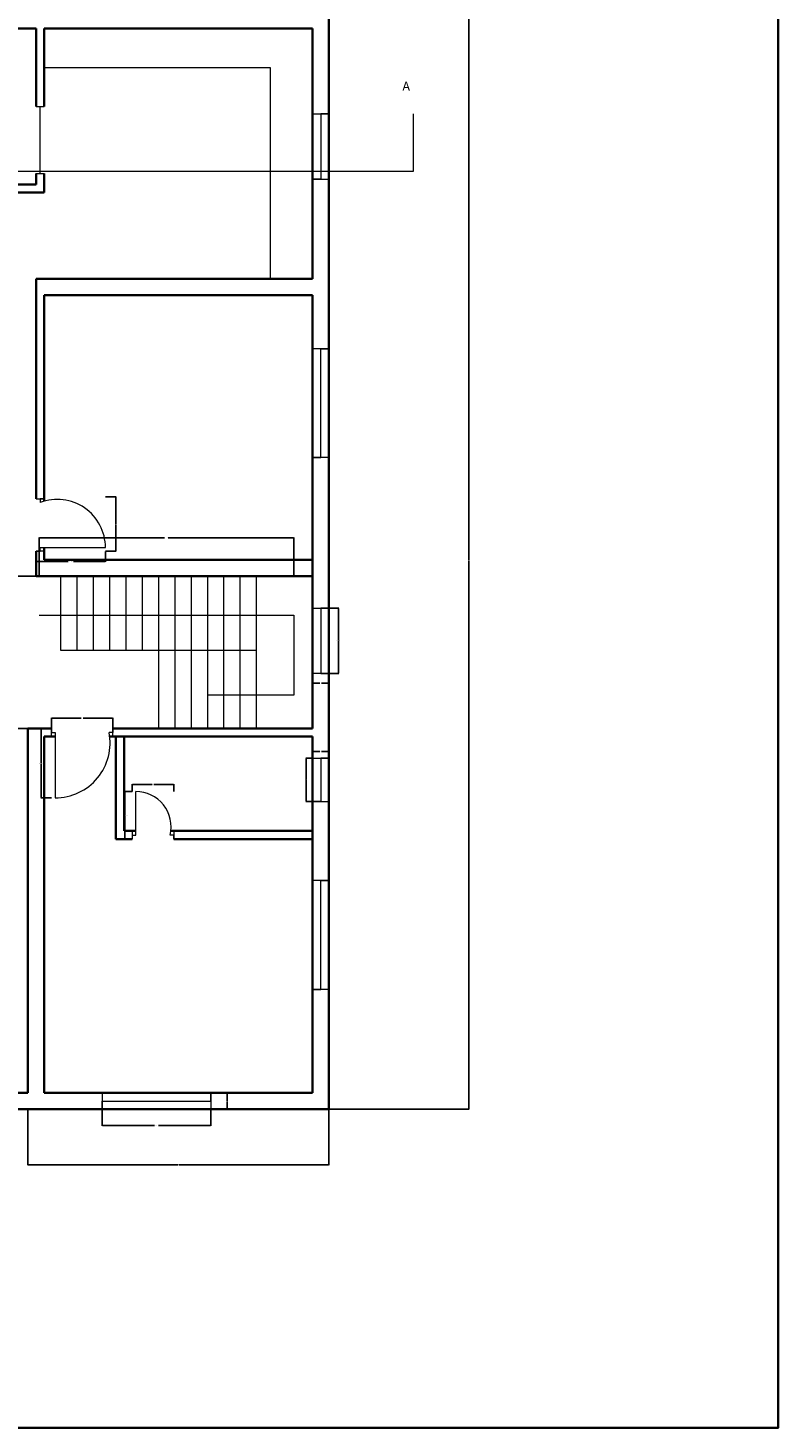
# Model space of a CAD drawing. Units: inches. Extents: x 1152 to 2588, y 1459 to 2618.
# Tile 16 of 17: x 2174 to 2588, y 1459 to 2231. Entities that reach past the tile are written whole.
import ezdxf

# ---------------------------------------------------------------- set-up
doc = ezdxf.new("R2010")
doc.units = ezdxf.units.IN
for name, color, linetype, lineweight in [('A-ANNO-DIMS', 2, 'Continuous', 18), ('A-ANNO-SYMB', 3, 'Continuous', 18), ('A-ANNO-TTLB', 7, 'Continuous', 35), ('A-DOOR', 4, 'Continuous', 18), ('A-FLOR-CASE', 30, 'Continuous', 18), ('A-FLOR-STRS', 3, 'Continuous', 18), ('A-GLAZ', 4, 'Continuous', 18), ('A-WALL', 7, 'Continuous', 35)]:
    doc.layers.add(name, color=color, linetype=linetype, lineweight=lineweight)
doc.styles.get("Standard").update_dxf_attribs({"font": 'arial.ttf'})
doc.dimstyles.get("Standard").update_dxf_attribs({"dimtxt": 0.18, "dimasz": 0.18, "dimexe": 0.18, "dimexo": 0.0625, "dimgap": 0.09, "dimtad": 0, "dimtih": 1, "dimtoh": 1, "dimdec": 4, "dimzin": 0, "dimdsep": 46, "dimtxsty": 'Standard', "dimcen": 0.09, "dimadec": 0, "dimazin": 0, "dimtfac": 1, "dimtdec": 4, "dimtofl": 0, "dimtmove": 0, "dimatfit": 3, "dimfxl": 1, "dimtolj": 1, "dimtzin": 0, "dimarcsym": 0})

# ---------------------------------------------------------------- blocks, each defined once
blk = doc.blocks.new('DOOR-24-ENSUITE')
for p, q in [((2, 2.25), (2, 26.25)), ((0, 4.5), (0, 0)), ((0, 2.25), (2, 2.25)), ((23, 2.25), (21, 2.25)), ((23, 4.5), (23, 0)), ((23, 0), (23, 2.25)), ((23, 2.25), (23, 2.25)), ((0, 0), (0, 0))]:
    blk.add_line(p, q)
blk.add_arc((2, 6.73), 19.52, 346.72099, 90)
blk = doc.blocks.new('DOOR-36-STORE')
for p, q in [((0, 28.88), (4.5, 28.88)), ((4.5, 28.88), (2.25, 28.88)), ((2.25, 28.88), (2.25, 26.88)), ((4.5, 0), (0, 0)), ((0, 0), (2.25, 0)), ((2.25, 0), (2.25, 2)), ((2.25, 2), (38.25, 2))]:
    blk.add_line(p, q)
blk.add_arc((11.65, 2), 26.6, 0, 110.70701)
blk = doc.blocks.new('DOOR-36-HALL')
for p, q in [((0, 33.75), (0, 38.25)), ((0, 38.25), (0, 36)), ((0, 36), (2, 36)), ((2, 36), (2, 0)), ((33.77, 36), (31.77, 36)), ((33.77, 33.75), (33.77, 38.25)), ((33.77, 38.25), (33.77, 36))]:
    blk.add_line(p, q)
blk.add_arc((2, 30.31), 30.31, 270, 10.81625)
blk = doc.blocks.new('DOOR-STORE-OPENING')
for p, q in [((0, 36.9), (4.5, 36.9)), ((2.25, 0), (2.25, 36.9)), ((0, 0), (4.5, 0))]:
    blk.add_line(p, q)
blk = doc.blocks.new('WIN-60-EXT')
for p, q in [((0, 9), (0, 0)), ((60, 4.5), (60, 9)), ((60, 9), (60, 0)), ((0, 0), (0, 4.5)), ((0, 4.5), (60, 4.5))]:
    blk.add_line(p, q)
blk = doc.blocks.new('WIN-36')
for p, q in [((0, 36), (9, 36)), ((9, 36), (4.5, 36)), ((4.5, 36), (4.5, 0)), ((4.5, 0), (0, 0)), ((0, 0), (9, 0))]:
    blk.add_line(p, q)
blk = doc.blocks.new('WIN-24-BATH-EAST')
for p, q in [((0, 24), (9, 24)), ((9, 24), (4.5, 24)), ((4.5, 24), (4.5, 0)), ((4.5, 0), (0, 0)), ((0, 0), (9, 0))]:
    blk.add_line(p, q)
blk = doc.blocks.new('WIN-36-STAIR')
for p, q in [((0, 36), (9, 36)), ((9, 36), (4.5, 36)), ((4.5, 36), (4.5, 0)), ((9, 0), (0, 0)), ((4.5, 0), (9, 0))]:
    blk.add_line(p, q)
blk = doc.blocks.new('STAIR-RETURN')
for p, q in [((12.04, 42.95), (12.04, 84)), ((21.04, 42.95), (21.04, 84)), ((30.04, 42.95), (30.04, 84)), ((39.04, 42.95), (39.04, 84)), ((48.04, 42.95), (48.04, 84)), ((57.04, 42.95), (57.04, 84)), ((66.04, 0), (66.04, 84)), ((75.04, 0), (75.04, 84)), ((84.04, 0), (84.04, 84)), ((93.04, 0), (93.04, 84)), ((102.04, 0), (102.04, 84)), ((111.04, 0), (111.04, 84)), ((120.04, 0), (120.04, 84)), ((0, 62.54), (140.6, 62.54)), ((140.6, 62.54), (140.6, 18.44)), ((120.04, 42.95), (12.04, 42.95)), ((140.6, 18.44), (93.04, 18.44))]:
    blk.add_line(p, q)
blk = doc.blocks.new('COUNTER-KITCHEN-L')
for p, q in [((0, 116.5), (124.66, 116.5)), ((124.66, 116.5), (124.66, 0))]:
    blk.add_line(p, q)
blk = doc.blocks.new('*D26')
at = {"layer": 'A-ANNO-DIMS', "color": 0, "lineweight": -2, "transparency": 16777216}
for p, q in [((2214.75, 1634.98), (2214.75, 1625.87)), ((2274.75, 1634.98), (2274.75, 1625.87)), ((2214.93, 1626.05), (2243.6, 1626.05)), ((2274.57, 1626.05), (2245.9, 1626.05))]:
    blk.add_line(p, q, dxfattribs=at)
at = {"layer": 'A-ANNO-DIMS', "color": 0, "transparency": 16777216}
for points in [[(2214.93, 1626.08), (2214.93, 1626.02), (2214.75, 1626.05)], [(2274.57, 1626.08), (2274.57, 1626.02), (2274.75, 1626.05)]]:
    blk.add_solid(points, dxfattribs=at)
at = {"layer": 'Defpoints', "color": 0, "transparency": 16777216}
for p in [(2214.75, 1635.05), (2274.75, 1635.05), (2274.75, 1626.05)]:
    blk.add_point(p, dxfattribs=at)
at = {"layer": 'A-ANNO-DIMS', "color": 0, "transparency": 16777216, "insert": (2244.75, 1626.05), "char_height": 0.18, "attachment_point": 5}
blk.add_mtext('\\A1;EXT. WIN. 60 TYP.', dxfattribs=at)
blk = doc.blocks.new('*D27')
at = {"layer": 'A-ANNO-DIMS', "color": 0, "lineweight": -2, "transparency": 16777216}
for p, q in [((2274.81, 1644.05), (2283.93, 1644.05)), ((2283.75, 1643.87), (2283.75, 1639.73)), ((2283.75, 1635.23), (2283.75, 1639.36)), ((2274.81, 1635.05), (2283.93, 1635.05))]:
    blk.add_line(p, q, dxfattribs=at)
at = {"layer": 'A-ANNO-DIMS', "color": 0, "transparency": 16777216}
for points in [[(2283.72, 1643.87), (2283.78, 1643.87), (2283.75, 1644.05)], [(2283.72, 1635.23), (2283.78, 1635.23), (2283.75, 1635.05)]]:
    blk.add_solid(points, dxfattribs=at)
at = {"layer": 'Defpoints', "color": 0, "transparency": 16777216}
for p in [(2274.75, 1644.05), (2283.75, 1644.05), (2274.75, 1635.05)]:
    blk.add_point(p, dxfattribs=at)
at = {"layer": 'A-ANNO-DIMS', "color": 0, "transparency": 16777216, "insert": (2283.75, 1639.55), "char_height": 0.18, "attachment_point": 5}
blk.add_mtext('\\A1;9 TYP.', dxfattribs=at)
blk = doc.blocks.new('*D38')
at = {"layer": 'A-ANNO-DIMS', "color": 0, "lineweight": -2, "transparency": 16777216}
for p, q in [((2231.28, 1810.3), (2227.22, 1810.3)), ((2227.4, 1810.12), (2227.4, 1797.35)), ((2227.4, 1784.23), (2227.4, 1796.99)), ((2231.28, 1784.05), (2227.22, 1784.05))]:
    blk.add_line(p, q, dxfattribs=at)
at = {"layer": 'A-ANNO-DIMS', "color": 0, "transparency": 16777216}
for points in [[(2227.37, 1810.12), (2227.43, 1810.12), (2227.4, 1810.3)], [(2227.37, 1784.23), (2227.43, 1784.23), (2227.4, 1784.05)]]:
    blk.add_solid(points, dxfattribs=at)
at = {"layer": 'Defpoints', "color": 0, "transparency": 16777216}
for p in [(2227.4, 1810.3), (2231.34, 1810.3), (2231.34, 1784.05)]:
    blk.add_point(p, dxfattribs=at)
at = {"layer": 'A-ANNO-DIMS', "color": 0, "transparency": 16777216, "insert": (2227.4, 1797.17), "char_height": 0.18, "attachment_point": 5}
blk.add_mtext('\\A1;ENSUITE DOOR 26 TYP.', dxfattribs=at)
blk = doc.blocks.new('*D39')
at = {"layer": 'A-ANNO-DIMS', "color": 0, "lineweight": -2, "transparency": 16777216}
for p, q in [((2231.34, 1810.36), (2231.34, 1814.41)), ((2231.52, 1814.23), (2242.31, 1814.23)), ((2254.15, 1814.23), (2243.36, 1814.23)), ((2254.33, 1810.36), (2254.33, 1814.41))]:
    blk.add_line(p, q, dxfattribs=at)
at = {"layer": 'A-ANNO-DIMS', "color": 0, "transparency": 16777216}
for points in [[(2231.52, 1814.26), (2231.52, 1814.2), (2231.34, 1814.23)], [(2254.15, 1814.26), (2254.15, 1814.2), (2254.33, 1814.23)]]:
    blk.add_solid(points, dxfattribs=at)
at = {"layer": 'Defpoints', "color": 0, "transparency": 16777216}
for p in [(2254.33, 1814.23), (2231.34, 1810.3), (2254.33, 1810.3)]:
    blk.add_point(p, dxfattribs=at)
at = {"layer": 'A-ANNO-DIMS', "color": 0, "transparency": 16777216, "insert": (2242.84, 1814.23), "char_height": 0.18, "attachment_point": 5}
blk.add_mtext('\\A1;23 TYP.', dxfattribs=at)
blk = doc.blocks.new('*D46')
at = {"layer": 'A-ANNO-DIMS', "color": 0, "lineweight": -2, "transparency": 16777216}
for p, q in [((2178.38, 1942.71), (2178.38, 1936.85)), ((2216.63, 1942.71), (2216.63, 1936.85)), ((2178.56, 1937.03), (2196.1, 1937.03)), ((2216.45, 1937.03), (2198.92, 1937.03))]:
    blk.add_line(p, q, dxfattribs=at)
at = {"layer": 'A-ANNO-DIMS', "color": 0, "transparency": 16777216}
for points in [[(2178.56, 1937.06), (2178.56, 1937), (2178.38, 1937.03)], [(2216.45, 1937.06), (2216.45, 1937), (2216.63, 1937.03)]]:
    blk.add_solid(points, dxfattribs=at)
at = {"layer": 'Defpoints', "color": 0, "transparency": 16777216}
for p in [(2178.38, 1942.77), (2216.63, 1942.77), (2216.63, 1937.03)]:
    blk.add_point(p, dxfattribs=at)
at = {"layer": 'A-ANNO-DIMS', "color": 0, "transparency": 16777216, "insert": (2197.51, 1937.03), "char_height": 0.18, "attachment_point": 5}
blk.add_mtext('\\A1;STORE DOOR 38 TYP.', dxfattribs=at)
blk = doc.blocks.new('*D47')
at = {"layer": 'A-ANNO-DIMS', "color": 0, "lineweight": -2, "transparency": 16777216}
for p, q in [((2216.7, 1972.74), (2222.55, 1972.74)), ((2222.37, 1972.56), (2222.37, 1957.94)), ((2222.37, 1942.95), (2222.37, 1957.57)), ((2216.7, 1942.77), (2222.55, 1942.77))]:
    blk.add_line(p, q, dxfattribs=at)
at = {"layer": 'A-ANNO-DIMS', "color": 0, "transparency": 16777216}
for points in [[(2222.34, 1972.56), (2222.4, 1972.56), (2222.37, 1972.74)], [(2222.34, 1942.95), (2222.4, 1942.95), (2222.37, 1942.77)]]:
    blk.add_solid(points, dxfattribs=at)
at = {"layer": 'Defpoints', "color": 0, "transparency": 16777216}
for p in [(2216.63, 1972.74), (2222.37, 1972.74), (2216.63, 1942.77)]:
    blk.add_point(p, dxfattribs=at)
at = {"layer": 'A-ANNO-DIMS', "color": 0, "transparency": 16777216, "insert": (2222.37, 1957.76), "char_height": 0.18, "attachment_point": 5}
blk.add_mtext('\\A1;30 TYP.', dxfattribs=at)
blk = doc.blocks.new('*D48')
at = {"layer": 'A-ANNO-DIMS', "color": 0, "lineweight": -2, "transparency": 16777216}
for p, q in [((2186.81, 1845.05), (2180.95, 1845.05)), ((2181.13, 1844.87), (2181.13, 1826.1)), ((2181.13, 1806.98), (2181.13, 1825.74)), ((2186.81, 1806.8), (2180.95, 1806.8))]:
    blk.add_line(p, q, dxfattribs=at)
at = {"layer": 'A-ANNO-DIMS', "color": 0, "transparency": 16777216}
for points in [[(2181.1, 1844.87), (2181.16, 1844.87), (2181.13, 1845.05)], [(2181.1, 1806.98), (2181.16, 1806.98), (2181.13, 1806.8)]]:
    blk.add_solid(points, dxfattribs=at)
at = {"layer": 'Defpoints', "color": 0, "transparency": 16777216}
for p in [(2181.13, 1845.05), (2186.87, 1845.05), (2186.87, 1806.8)]:
    blk.add_point(p, dxfattribs=at)
at = {"layer": 'A-ANNO-DIMS', "color": 0, "transparency": 16777216, "insert": (2181.13, 1825.92), "char_height": 0.18, "attachment_point": 5}
blk.add_mtext('\\A1;HALL DOOR 38 TYP.', dxfattribs=at)
blk = doc.blocks.new('*D49')
at = {"layer": 'A-ANNO-DIMS', "color": 0, "lineweight": -2, "transparency": 16777216}
for p, q in [((2186.87, 1845.11), (2186.87, 1850.96)), ((2187.05, 1850.78), (2203.23, 1850.78)), ((2220.46, 1850.78), (2204.29, 1850.78)), ((2220.64, 1845.11), (2220.64, 1850.96))]:
    blk.add_line(p, q, dxfattribs=at)
at = {"layer": 'A-ANNO-DIMS', "color": 0, "transparency": 16777216}
for points in [[(2187.05, 1850.81), (2187.05, 1850.75), (2186.87, 1850.78)], [(2220.46, 1850.81), (2220.46, 1850.75), (2220.64, 1850.78)]]:
    blk.add_solid(points, dxfattribs=at)
at = {"layer": 'Defpoints', "color": 0, "transparency": 16777216}
for p in [(2186.87, 1845.05), (2220.64, 1850.78), (2220.64, 1845.05)]:
    blk.add_point(p, dxfattribs=at)
at = {"layer": 'A-ANNO-DIMS', "color": 0, "transparency": 16777216, "insert": (2203.76, 1850.78), "char_height": 0.18, "attachment_point": 5}
blk.add_mtext('\\A1;34 TYP.', dxfattribs=at)
blk = doc.blocks.new('*D58')
at = {"layer": 'A-ANNO-DIMS', "color": 0, "lineweight": -2, "transparency": 16777216}
for p, q in [((2330.82, 1828.76), (2327.1, 1828.76)), ((2327.28, 1828.58), (2327.28, 1816.94)), ((2327.28, 1804.94), (2327.28, 1816.58)), ((2330.82, 1804.76), (2327.1, 1804.76))]:
    blk.add_line(p, q, dxfattribs=at)
at = {"layer": 'A-ANNO-DIMS', "color": 0, "transparency": 16777216}
for points in [[(2327.25, 1828.58), (2327.31, 1828.58), (2327.28, 1828.76)], [(2327.25, 1804.94), (2327.31, 1804.94), (2327.28, 1804.76)]]:
    blk.add_solid(points, dxfattribs=at)
at = {"layer": 'Defpoints', "color": 0, "transparency": 16777216}
for p in [(2327.28, 1828.76), (2330.88, 1828.76), (2330.88, 1804.76)]:
    blk.add_point(p, dxfattribs=at)
at = {"layer": 'A-ANNO-DIMS', "color": 0, "transparency": 16777216, "insert": (2327.28, 1816.76), "char_height": 0.18, "attachment_point": 5}
blk.add_mtext('\\A1;WIN. 24 TYP.', dxfattribs=at)
blk = doc.blocks.new('*D59')
at = {"layer": 'A-ANNO-DIMS', "color": 0, "lineweight": -2, "transparency": 16777216}
for p, q in [((2330.88, 1828.82), (2330.88, 1832.54)), ((2331.06, 1832.36), (2334.93, 1832.36)), ((2339.7, 1832.36), (2335.84, 1832.36)), ((2339.88, 1828.82), (2339.88, 1832.54))]:
    blk.add_line(p, q, dxfattribs=at)
at = {"layer": 'A-ANNO-DIMS', "color": 0, "transparency": 16777216}
for points in [[(2331.06, 1832.39), (2331.06, 1832.33), (2330.88, 1832.36)], [(2339.7, 1832.39), (2339.7, 1832.33), (2339.88, 1832.36)]]:
    blk.add_solid(points, dxfattribs=at)
at = {"layer": 'Defpoints', "color": 0, "transparency": 16777216}
for p in [(2339.88, 1832.36), (2330.88, 1828.76), (2339.88, 1828.76)]:
    blk.add_point(p, dxfattribs=at)
at = {"layer": 'A-ANNO-DIMS', "color": 0, "transparency": 16777216, "insert": (2335.38, 1832.36), "char_height": 0.18, "attachment_point": 5}
blk.add_mtext('\\A1;9 TYP.', dxfattribs=at)
blk = doc.blocks.new('*D62')
at = {"layer": 'A-ANNO-DIMS', "color": 0, "lineweight": -2, "transparency": 16777216}
for p, q in [((2339.95, 1911.36), (2345.46, 1911.36)), ((2345.28, 1911.18), (2345.28, 1893.54)), ((2345.28, 1875.54), (2345.28, 1893.17)), ((2339.95, 1875.36), (2345.46, 1875.36))]:
    blk.add_line(p, q, dxfattribs=at)
at = {"layer": 'A-ANNO-DIMS', "color": 0, "transparency": 16777216}
for points in [[(2345.25, 1911.18), (2345.31, 1911.18), (2345.28, 1911.36)], [(2345.25, 1875.54), (2345.31, 1875.54), (2345.28, 1875.36)]]:
    blk.add_solid(points, dxfattribs=at)
at = {"layer": 'Defpoints', "color": 0, "transparency": 16777216}
for p in [(2339.88, 1911.36), (2345.28, 1911.36), (2339.88, 1875.36)]:
    blk.add_point(p, dxfattribs=at)
at = {"layer": 'A-ANNO-DIMS', "color": 0, "transparency": 16777216, "insert": (2345.28, 1893.36), "char_height": 0.18, "attachment_point": 5}
blk.add_mtext('\\A1;STAIR WIN. 36 TYP.', dxfattribs=at)
blk = doc.blocks.new('*D63')
at = {"layer": 'A-ANNO-DIMS', "color": 0, "lineweight": -2, "transparency": 16777216}
for p, q in [((2330.88, 1875.29), (2330.88, 1869.78)), ((2331.06, 1869.96), (2334.93, 1869.96)), ((2339.7, 1869.96), (2335.84, 1869.96)), ((2339.88, 1875.29), (2339.88, 1869.78))]:
    blk.add_line(p, q, dxfattribs=at)
at = {"layer": 'A-ANNO-DIMS', "color": 0, "transparency": 16777216}
for points in [[(2331.06, 1869.99), (2331.06, 1869.93), (2330.88, 1869.96)], [(2339.7, 1869.99), (2339.7, 1869.93), (2339.88, 1869.96)]]:
    blk.add_solid(points, dxfattribs=at)
at = {"layer": 'Defpoints', "color": 0, "transparency": 16777216}
for p in [(2330.88, 1875.36), (2339.88, 1875.36), (2339.88, 1869.96)]:
    blk.add_point(p, dxfattribs=at)
at = {"layer": 'A-ANNO-DIMS', "color": 0, "transparency": 16777216, "insert": (2335.38, 1869.96), "char_height": 0.18, "attachment_point": 5}
blk.add_mtext('\\A1;9 TYP.', dxfattribs=at)
blk = doc.blocks.new('*D66')
at = {"layer": 'A-ANNO-DIMS', "color": 0, "lineweight": -2, "transparency": 16777216}
for p, q in [((2179.99, 1929.11), (2179.99, 1950.32)), ((2180.17, 1950.14), (2249.29, 1950.14)), ((2320.41, 1950.14), (2251.29, 1950.14)), ((2320.59, 1929.11), (2320.59, 1950.32))]:
    blk.add_line(p, q, dxfattribs=at)
at = {"layer": 'A-ANNO-DIMS', "color": 0, "transparency": 16777216}
for points in [[(2180.17, 1950.17), (2180.17, 1950.11), (2179.99, 1950.14)], [(2320.41, 1950.17), (2320.41, 1950.11), (2320.59, 1950.14)]]:
    blk.add_solid(points, dxfattribs=at)
at = {"layer": 'Defpoints', "color": 0, "transparency": 16777216}
for p in [(2320.59, 1950.14), (2179.99, 1929.05), (2320.59, 1929.05)]:
    blk.add_point(p, dxfattribs=at)
at = {"layer": 'A-ANNO-DIMS', "color": 0, "transparency": 16777216, "insert": (2250.29, 1950.14), "char_height": 0.18, "attachment_point": 5}
blk.add_mtext('\\A1;STAIR 141 TYP.', dxfattribs=at)
blk = doc.blocks.new('*D67')
at = {"layer": 'A-ANNO-DIMS', "color": 0, "lineweight": -2, "transparency": 16777216}
for p, q in [((2179.93, 1929.05), (2158.72, 1929.05)), ((2158.9, 1928.87), (2158.9, 1887.23)), ((2158.9, 1845.23), (2158.9, 1886.86)), ((2179.93, 1845.05), (2158.72, 1845.05))]:
    blk.add_line(p, q, dxfattribs=at)
at = {"layer": 'A-ANNO-DIMS', "color": 0, "transparency": 16777216}
for points in [[(2158.87, 1928.87), (2158.93, 1928.87), (2158.9, 1929.05)], [(2158.87, 1845.23), (2158.93, 1845.23), (2158.9, 1845.05)]]:
    blk.add_solid(points, dxfattribs=at)
at = {"layer": 'Defpoints', "color": 0, "transparency": 16777216}
for p in [(2158.9, 1929.05), (2179.99, 1929.05), (2179.99, 1845.05)]:
    blk.add_point(p, dxfattribs=at)
at = {"layer": 'A-ANNO-DIMS', "color": 0, "transparency": 16777216, "insert": (2158.9, 1887.05), "char_height": 0.18, "attachment_point": 5}
blk.add_mtext('\\A1;84 TYP.', dxfattribs=at)
blk = doc.blocks.new('*D78')
at = {"layer": 'A-ANNO-DIMS', "color": 0, "lineweight": -2, "transparency": 16777216}
for p, q in [((2339.95, 2240.05), (2417.36, 2240.05)), ((2417.18, 2239.87), (2417.18, 1937.73)), ((2417.18, 1635.23), (2417.18, 1937.36)), ((2339.95, 1635.05), (2417.36, 1635.05))]:
    blk.add_line(p, q, dxfattribs=at)
at = {"layer": 'A-ANNO-DIMS', "color": 0, "transparency": 16777216}
for points in [[(2417.15, 2239.87), (2417.21, 2239.87), (2417.18, 2240.05)], [(2417.15, 1635.23), (2417.21, 1635.23), (2417.18, 1635.05)]]:
    blk.add_solid(points, dxfattribs=at)
at = {"layer": 'Defpoints', "color": 0, "transparency": 16777216}
for p in [(2339.88, 2240.05), (2417.18, 2240.05), (2339.88, 1635.05)]:
    blk.add_point(p, dxfattribs=at)
at = {"layer": 'A-ANNO-DIMS', "color": 0, "transparency": 16777216, "insert": (2417.18, 1937.55), "char_height": 0.18, "attachment_point": 5}
blk.add_mtext('\\A1;605', dxfattribs=at)
blk = doc.blocks.new('*D87')
at = {"layer": 'A-ANNO-DIMS', "color": 0, "lineweight": -2, "transparency": 16777216}
for p, q in [((2173.88, 1634.98), (2173.88, 1604.27)), ((2339.88, 1634.98), (2339.88, 1604.27)), ((2174.06, 1604.45), (2256.6, 1604.45)), ((2339.7, 1604.45), (2257.16, 1604.45))]:
    blk.add_line(p, q, dxfattribs=at)
at = {"layer": 'A-ANNO-DIMS', "color": 0, "transparency": 16777216}
for points in [[(2174.06, 1604.48), (2174.06, 1604.42), (2173.88, 1604.45)], [(2339.7, 1604.48), (2339.7, 1604.42), (2339.88, 1604.45)]]:
    blk.add_solid(points, dxfattribs=at)
at = {"layer": 'Defpoints', "color": 0, "transparency": 16777216}
for p in [(2173.88, 1635.05), (2339.88, 1635.05), (2339.88, 1604.45)]:
    blk.add_point(p, dxfattribs=at)
at = {"layer": 'A-ANNO-DIMS', "color": 0, "transparency": 16777216, "insert": (2256.88, 1604.45), "char_height": 0.18, "attachment_point": 5}
blk.add_mtext('\\A1;166', dxfattribs=at)

msp = doc.modelspace()

# ---------------------------------------------------------------- linework, layer by layer
at = {"layer": 'A-ANNO-SYMB'}
for p, q in [((2386.5775, 2152.3313), (2386.5775, 2183.955)), ((1847.169, 2152.3313), (2386.5775, 2152.3313))]:
    msp.add_line(p, q, dxfattribs=at)
at = {"layer": 'A-ANNO-TTLB'}
msp.add_lwpolyline([(1152.3215, 2617.6685), (2587.6987, 2617.6685), (2587.6987, 1459.3148), (1152.3215, 1459.3148)], close=True, dxfattribs=at)
at = {"layer": 'A-WALL'}
for p, q in [((2339.8841, 2240.0458), (2339.8841, 1635.0458)), ((2130.3841, 2231.0458), (2178.3841, 2231.0458)), ((2178.3841, 2231.0458), (2178.3841, 2188.0458)), ((2182.8841, 2231.0458), (2330.8841, 2231.0458)), ((2182.8841, 2231.0458), (2182.8841, 2188.0458)), ((2330.8841, 2231.0458), (2330.8841, 2093.0458)), ((2178.3841, 2151.1471), (2178.3841, 2145.0458)), ((2182.8841, 2151.1471), (2182.8841, 2140.5458)), ((2130.3841, 2145.0458), (2178.3841, 2145.0458)), ((2130.3841, 2140.5458), (2178.3841, 2140.5458)), ((2178.3841, 2140.5458), (2182.8841, 2140.5458)), ((2178.3841, 2093.0458), (2178.3841, 1971.6501)), ((2182.8841, 2093.0458), (2178.3841, 2093.0458)), ((2182.8841, 2093.0458), (2330.8841, 2093.0458)), ((2182.8841, 2084.0458), (2330.8841, 2084.0458)), ((2182.8841, 2084.0458), (2182.8841, 1970.3879)), ((2330.8841, 2084.0458), (2330.8841, 1845.0458)), ((2178.3841, 1942.7722), (2178.3841, 1929.0458)), ((2182.8841, 1944.7722), (2182.8841, 1938.0458)), ((2182.8841, 1938.0458), (2330.8841, 1938.0458)), ((2178.3841, 1929.0458), (2330.8841, 1929.0458)), ((2173.8841, 1845.0458), (2182.8841, 1845.0458)), ((2173.8841, 1840.5831), (2173.8841, 1845.0458)), ((2182.8841, 1845.0458), (2186.8711, 1845.0458)), ((2220.6443, 1845.0458), (2330.8841, 1845.0458)), ((2173.8841, 1644.0458), (2173.8841, 1840.5831)), ((2182.8841, 1840.5458), (2188.8711, 1840.5458)), ((2182.8841, 1840.5458), (2182.8841, 1644.0458)), ((2218.9872, 1840.5458), (2330.8841, 1840.5458)), ((2226.8841, 1840.5458), (2222.3841, 1840.5458)), ((2222.3841, 1840.5458), (2222.3841, 1788.5458)), ((2226.8841, 1788.5458), (2226.8841, 1840.5458)), ((2330.8841, 1840.5458), (2330.8841, 1644.0458)), ((2330.8841, 1840.5458), (2330.8841, 1788.5458)), ((2222.3841, 1788.5458), (2222.3841, 1784.0458)), ((2222.3841, 1784.0458), (2231.3375, 1784.0458)), ((2233.3375, 1788.5458), (2226.8841, 1788.5458)), ((2330.8841, 1788.5458), (2252.7264, 1788.5458)), ((2254.3327, 1784.0458), (2330.8841, 1784.0458)), ((2073.5339, 1644.0458), (2173.8841, 1644.0458)), ((2182.8841, 1644.0458), (2330.8841, 1644.0458)), ((2075.5339, 1635.0458), (2339.8841, 1635.0458)), ((2182.8841, 1635.0458), (2173.8841, 1635.0458))]:
    msp.add_line(p, q, dxfattribs=at)

# ---------------------------------------------------------------- block references
at = {"layer": 'A-DOOR'}
for name, p in [('DOOR-STORE-OPENING', (2178.3846, 2151.147)), ('DOOR-36-STORE', (2178.3846, 1942.772)), ('DOOR-36-HALL', (2186.8716, 1806.796)), ('DOOR-24-ENSUITE', (2231.3376, 1784.046))]:
    msp.add_blockref(name, p, dxfattribs=at)
at = {"layer": 'A-FLOR-CASE'}
msp.add_blockref('COUNTER-KITCHEN-L', (2182.8846, 2093.046), dxfattribs=at)
at = {"layer": 'A-FLOR-STRS'}
msp.add_blockref('STAIR-RETURN', (2179.9916, 1845.046), dxfattribs=at)
at = {"layer": 'A-GLAZ'}
for name, p in [('WIN-36', (2330.8846, 2147.9727)), ('WIN-36-STAIR', (2330.8846, 1875.356)), ('WIN-24-BATH-EAST', (2330.8846, 1804.762)), ('WIN-60-EXT', (2214.7476, 1635.046))]:
    msp.add_blockref(name, p, dxfattribs=at)
at = {"layer": 'A-GLAZ', "extrusion": (0, 0, -1), "zscale": -1, "rotation": 90}
for p in [(-2330.8843, 1994.3846), (-2330.8843, 1701.1862)]:
    msp.add_blockref('WIN-60-EXT', p, dxfattribs=at)

# ---------------------------------------------------------------- texts
at = {"layer": 'A-ANNO-SYMB', "insert": (2380.4913, 2201.7342), "char_height": 5, "attachment_point": 1}
msp.add_mtext_dynamic_manual_height_columns('A', width=59.913594, gutter_width=12.5, heights=[0], dxfattribs=at)

# ---------------------------------------------------------------- dimensions: what is measured, and where the dimension line sits
at = {"layer": 'A-ANNO-DIMS'}
dim = msp.add_linear_dim(base=(2417.1775, 2240.0458), p1=(2339.8841, 1635.0458), p2=(2339.8841, 2240.0458), angle=90, dimstyle='Standard', override={"dimdec": 0, "dimlfac": 1, "dimrnd": 0, "dimzin": 0, "dimdsep": 46, "dimlunit": 2}, dxfattribs=at)
dim.commit()
dim.dimension.update_dxf_attribs({"geometry": '*D78', "text_midpoint": (2417.1775, 1937.5458)})
for base, p1, p2, text, picture, middle in [((2222.3716, 1972.7388), (2216.6341, 1942.7722), (2216.6341, 1972.7388), '<> TYP.', '*D47', (2222.3716, 1957.7555)), ((2158.9012, 1929.0458), (2179.9911, 1845.0458), (2179.9911, 1929.0458), '<> TYP.', '*D67', (2158.9012, 1887.0458)), ((2345.2841, 1911.3562), (2339.8841, 1875.3562), (2339.8841, 1911.3562), 'STAIR WIN. <> TYP.', '*D62', (2345.2841, 1893.3562)), ((2181.1336, 1845.0458), (2186.8711, 1806.7958), (2186.8711, 1845.0458), 'HALL DOOR <> TYP.', '*D48', (2181.1336, 1825.9208)), ((2327.2841, 1828.7619), (2330.8841, 1804.7619), (2330.8841, 1828.7619), 'WIN. <> TYP.', '*D58', (2327.2841, 1816.7619)), ((2227.4, 1810.2958), (2231.3375, 1784.0458), (2231.3375, 1810.2958), 'ENSUITE DOOR <> TYP.', '*D38', (2227.4, 1797.1708)), ((2283.7477, 1644.0458), (2274.7477, 1635.0458), (2274.7477, 1644.0458), '<> TYP.', '*D27', (2283.7477, 1639.5458))]:
    dim = msp.add_linear_dim(base=base, p1=p1, p2=p2, angle=90, text=text, dimstyle='Standard', override={"dimdec": 0, "dimlfac": 1, "dimrnd": 0, "dimzin": 0, "dimdsep": 46, "dimlunit": 2}, dxfattribs=at)
    dim.commit()
    dim.dimension.update_dxf_attribs({"geometry": picture, "text_midpoint": middle})
for base, p1, p2, text, picture, middle in [((2320.5901, 1950.1357), (2179.9911, 1929.0458), (2320.5901, 1929.0458), 'STAIR <> TYP.', '*D66', (2250.2906, 1950.1357)), ((2216.6341, 1937.0347), (2178.3841, 1942.7722), (2216.6341, 1942.7722), 'STORE DOOR <> TYP.', '*D46', (2197.5091, 1937.0347)), ((2339.8841, 1869.9562), (2330.8841, 1875.3562), (2339.8841, 1875.3562), '<> TYP.', '*D63', (2335.3841, 1869.9562)), ((2220.6443, 1850.7833), (2186.8711, 1845.0458), (2220.6443, 1845.0458), '<> TYP.', '*D49', (2203.7577, 1850.7833)), ((2339.8841, 1832.3619), (2330.8841, 1828.7619), (2339.8841, 1828.7619), '<> TYP.', '*D59', (2335.3841, 1832.3619)), ((2254.3327, 1814.2333), (2231.3375, 1810.2958), (2254.3327, 1810.2958), '<> TYP.', '*D39', (2242.8351, 1814.2333)), ((2274.7477, 1626.0458), (2214.7477, 1635.0458), (2274.7477, 1635.0458), 'EXT. WIN. <> TYP.', '*D26', (2244.7477, 1626.0458))]:
    dim = msp.add_linear_dim(base=base, p1=p1, p2=p2, text=text, dimstyle='Standard', override={"dimdec": 0, "dimlfac": 1, "dimrnd": 0, "dimzin": 0, "dimdsep": 46, "dimlunit": 2}, dxfattribs=at)
    dim.commit()
    dim.dimension.update_dxf_attribs({"geometry": picture, "text_midpoint": middle})
dim = msp.add_linear_dim(base=(2339.8841, 1604.4458), p1=(2173.8841, 1635.0458), p2=(2339.8841, 1635.0458), dimstyle='Standard', override={"dimdec": 0, "dimlfac": 1, "dimrnd": 0, "dimzin": 0, "dimdsep": 46, "dimlunit": 2}, dxfattribs=at)
dim.commit()
dim.dimension.update_dxf_attribs({"geometry": '*D87', "text_midpoint": (2256.8841, 1604.4458)})

doc.saveas('drawing.dxf')
